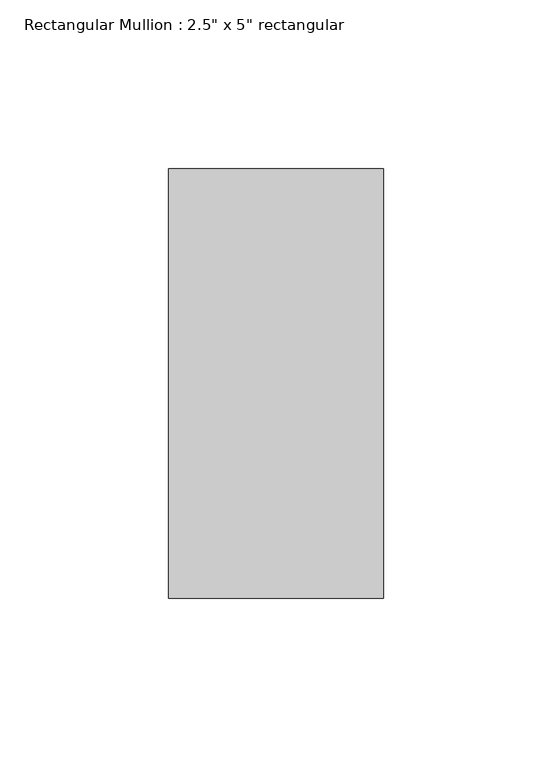
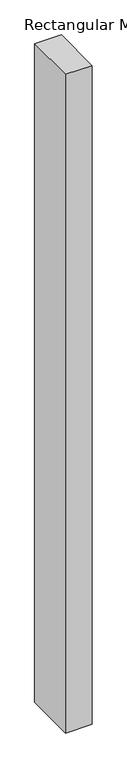
"""IFC4 building model written with IfcOpenShell, lengths in millimetres: member geometry."""

from ifc_helpers import new_model, si_unit, frame, origin, place, context, project, spatial, polyline, outline, extrude, source, transform, mapped, element, save


def member_f01f4494(model_context):
    return source(origin(), model_context, "Body", "SweptSolid", [
        extrude(outline(polyline([(31.75, 63.5), (31.75, -63.5), (-31.75, -63.5), (-31.75, 63.5), (31.75, 63.5)])), frame((0.0, 0.0, -1656.4112238), z_axis=(0.0, 0.0, 1.0), x_axis=(1.0, 0.0, 0.0)), (0.0, 0.0, 1.0), 1656.4112238),
    ])


if __name__ == "__main__":
    model = new_model("IFC4")
    model_context = context("Model", 3, world=origin())
    ifc_project = project(units=[si_unit("LENGTHUNIT", "METRE", prefix="MILLI")], contexts=[model_context])
    site = spatial("IfcSite", under=ifc_project)
    building = spatial("IfcBuilding", under=site)
    placement = place(None, origin())
    member_shape = member_f01f4494(model_context)
    element("IfcMember", 1, ObjectType="Rectangular Mullion : 2.5\" x 5\" rectangular", at=placement, inside=building, context=model_context, shape_type="MappedRepresentation", body=[
        mapped(member_shape, transform((0.0, 0.0, 0.0), x_axis=(1.0, 0.0, 0.0), y_axis=(0.0, 1.0, 0.0), z_axis=(0.0, 0.0, 1.0))),
    ])
    save(model, "model.ifc")

# Revit data of these elements
# Type "Rectangular Mullion : 2.5\" x 5\" rectangular"
#   built-in parameter 1007304 = 0.416667 (stored number, unit not read)
#   built-in parameter 1007301 = 0.104167 (stored number, unit not read)
#   built-in parameter 1007300 = 0.104167 (stored number, unit not read)
# Element 1 (IfcMember, "Rectangular Mullion : 2.5\" x 5\" rectangular")
#   Materials on its faces: "Aluminum"
# Materials
#   "Aluminum": class "Metal", colour RGB 247 247 247, transparency 0, Description = "Aluminum 6061", Cost = 0
